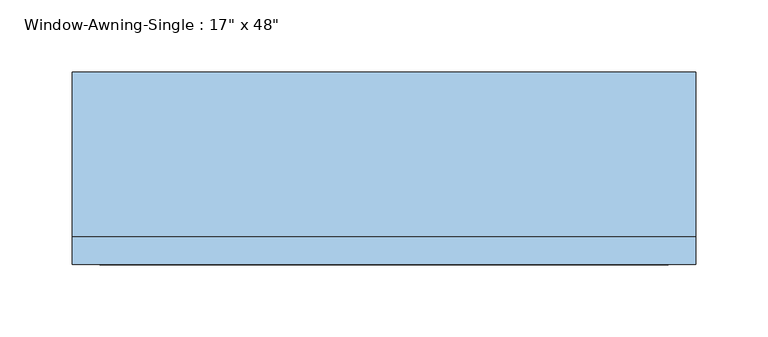
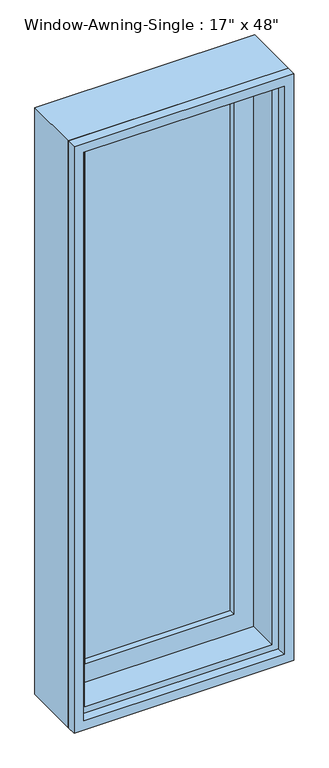
"""IFC4 building model written with IfcOpenShell, lengths in millimetres: window geometry."""

from ifc_helpers import new_model, si_unit, frame, origin, place, context, project, spatial, polyline, outline, extrude, faceted_brep, source, transform, mapped, element, save


def window_4630e4ac(model_context):
    return source(origin(), model_context, "Body", "SolidModel", [
        extrude(outline(polyline([(2133.6, -215.9), (914.4, -215.9), (914.4, 215.9), (2133.6, 215.9), (2133.6, -215.9)]), holes=[polyline([(2114.55, -196.85), (2114.55, 196.85), (933.45, 196.85), (933.45, -196.85), (2114.55, -196.85)])]), frame((0.0, -57.15, 0.0), z_axis=(0.0, 1.0, 0.0), x_axis=(0.0, 0.0, 1.0)), (0.0, 0.0, 1.0), 19.05),
        extrude(outline(polyline([(927.1, -203.2), (927.1, 203.2), (2120.9, 203.2), (2120.9, -203.2), (927.1, -203.2)]), holes=[polyline([(2063.75, -146.05), (2063.75, 146.05), (984.25, 146.05), (984.25, -146.05), (2063.75, -146.05)])]), frame((0.0, 25.4, 0.0), z_axis=(0.0, 1.0, 0.0), x_axis=(0.0, 0.0, 1.0)), (0.0, 0.0, 1.0), 44.45),
        extrude(outline(polyline([(146.05, 57.15), (146.05, 50.8), (-146.05, 50.8), (-146.05, 57.15), (146.05, 57.15)])), frame((0.0, 0.0, 984.25), z_axis=(0.0, 0.0, 1.0), x_axis=(1.0, 0.0, 0.0)), (0.0, 0.0, 1.0), 1079.5),
        extrude(outline(polyline([(146.05, 44.45), (146.05, 38.1), (-146.05, 38.1), (-146.05, 44.45), (146.05, 44.45)])), frame((0.0, 0.0, 984.25), z_axis=(0.0, 0.0, 1.0), x_axis=(1.0, 0.0, 0.0)), (0.0, 0.0, 1.0), 1079.5),
        faceted_brep([(203.2, 25.4, 927.1), (203.2, 76.2, 927.1), (-203.2, 76.2, 927.1), (-203.2, 25.4, 927.1), (184.15, -38.1, 946.15), (184.15, 25.4, 946.15), (-184.15, 25.4, 946.15), (-184.15, -38.1, 946.15), (215.9, 76.2, 914.4), (215.9, -38.1, 914.4), (-215.9, -38.1, 914.4), (-215.9, 76.2, 914.4), (-203.2, 76.2, 2120.9), (-203.2, 25.4, 2120.9), (-184.15, 25.4, 2101.85), (-184.15, -38.1, 2101.85), (-215.9, -38.1, 2133.6), (-215.9, 76.2, 2133.6), (203.2, 76.2, 2120.9), (203.2, 25.4, 2120.9), (184.15, 25.4, 2101.85), (184.15, -38.1, 2101.85), (215.9, -38.1, 2133.6), (215.9, 76.2, 2133.6)], [[[0, 1, 2, 3]], [[4, 5, 6, 7]], [[8, 9, 10, 11]], [[3, 2, 12, 13]], [[7, 6, 14, 15]], [[11, 10, 16, 17]], [[13, 12, 18, 19]], [[15, 14, 20, 21]], [[17, 16, 22, 23]], [[11, 17, 23, 8], [1, 18, 12, 2]], [[19, 18, 1, 0]], [[3, 13, 19, 0], [5, 20, 14, 6]], [[21, 20, 5, 4]], [[9, 22, 16, 10], [7, 15, 21, 4]], [[23, 22, 9, 8]]]),
    ])


if __name__ == "__main__":
    model = new_model("IFC4")
    model_context = context("Model", 3, world=origin())
    ifc_project = project(units=[si_unit("LENGTHUNIT", "METRE", prefix="MILLI")], contexts=[model_context])
    site = spatial("IfcSite", under=ifc_project)
    building = spatial("IfcBuilding", under=site)
    placement = place(None, origin())
    window_shape = window_4630e4ac(model_context)
    element("IfcWindow", 1, ObjectType="Window-Awning-Single : 17\" x 48\"", at=placement, inside=building, context=model_context, shape_type="MappedRepresentation", body=[
        mapped(window_shape, transform((0.0, 0.0, 0.0), x_axis=(1.0, 0.0, 0.0), y_axis=(0.0, 1.0, 0.0), z_axis=(0.0, 0.0, 1.0))),
    ])
    save(model, "model.ifc")

# Revit data of these elements
# Type "Window-Awning-Single : 17\" x 48\""
#   Type Mark = "27"
#   Fire Rating = "0.5h"
#   Assembly Code = "B2020100"
#   Analytic Construction = "Double glazing - domestic"
#   Window Inset [instance default] = 0' - 0"
#   Wall Thickness [instance default] = 0' - 6"
#   Visual Light Transmittance = 0.81
#   Thermal Resistance (R) = 1.8146 (h·ft²·°F)/BTU
#   Solar Heat Gain Coefficient = 0.76
#   Rough Width = 1' - 5 1/2"
#   Rough Height = 4' - 0 1/2"
#   Interior Wall Closure [instance default] = 0' - 2 1/4"
#   Height = 4' - 0"
#   Heat Transfer Coefficient (U) = 0.5511 BTU/(h·ft²·°F)
#   Frame Extension [instance default] = 0' - 0 1/4"
#   Exterior Wall Closure [instance default] = 0' - 1 1/4"
#   Extension Jamb [instance default] = 0' - 2 1/4"
#   Default Sill Height = 3' - 0"
#   Width = 1' - 5"
#   Muntin Visibility = yes
#   Interior Trim Visibility [instance default] = yes
#   Exterior Trim Visibility [instance default] = yes
#   Extension Jamb Visibility [instance default] = yes
#   Muntin Pattern = Muntin Pattern_2x2 : Muntin Pattern_2x2
#   Interior Trim Material = Wood - Stained
#   Interior Trim = Trim-Window-Interior-Flat : Picture Frame
#   Interior Frame Material = Wood - Stained
#   Glass Panel Material = Glass
#   Exterior Trim Material = Clad - White
#   Exterior Trim = Trim-Window-Exterior-Flat : with Sill
#   Exterior Frame Material = Clad - White
#   Wall Closure = (empty or 0)
# Element 1 (IfcWindow, "Window-Awning-Single : 17\" x 48\"")
#   Wall Thickness = 0' - 4 1/2"
#   Extension Jamb = 0' - 0 3/4"
#   Materials on its faces: "Wood - Stained", "Glass", "Clad - White"
# Materials
#   "Wood - Stained": class "Wood", colour RGB 224 178 126, transparency 0, Cost = 0
#   "Glass": class "Glass", colour RGB 0 128 192, transparency 0.75, Description = "Soda Lime Glass", Cost = 0
#   "Clad - White": class "Wood", colour RGB 242 242 238, transparency 0, Cost = 0
